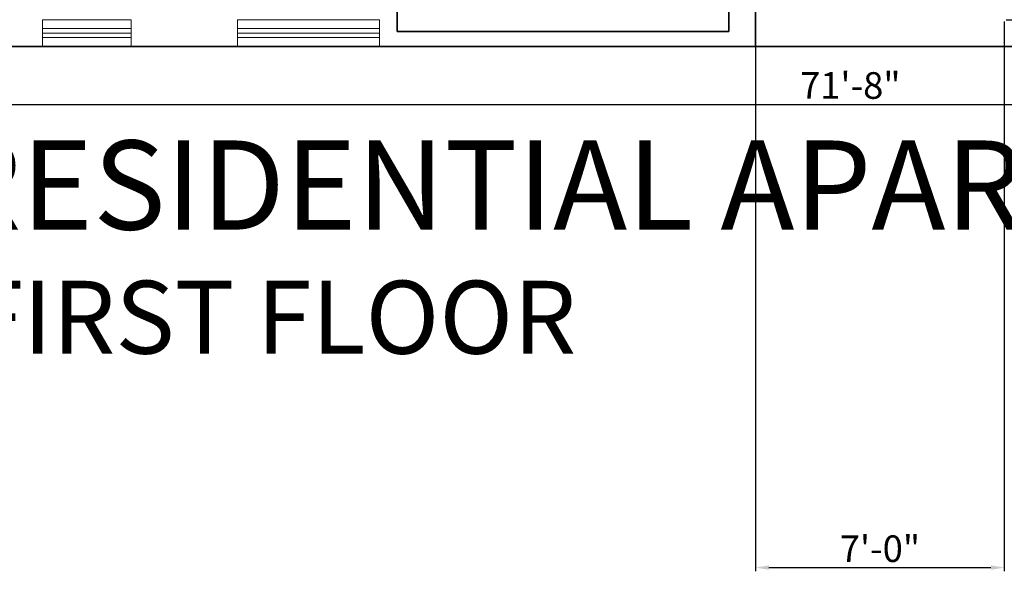
# Model space of a CAD drawing. Units: inches. Extents: x 2081 to 4786, y 1256 to 3802.
# Tile 2 of 7: x 2352 to 2685, y 1256 to 1442. Entities that reach past the tile are written whole.
import ezdxf

# ---------------------------------------------------------------- set-up
doc = ezdxf.new("R2010")
doc.units = ezdxf.units.IN
for name, color, linetype, lineweight in [('A-ANNO-DIMS', 18, 'Continuous', 18), ('A-ANNO-TITL', 18, 'Continuous', 35), ('A-GLAZ', 11, 'Continuous', 18), ('A-WALL', 7, 'Continuous', 35)]:
    doc.layers.add(name, color=color, linetype=linetype, lineweight=lineweight)
doc.styles.get("Standard").update_dxf_attribs({"font": 'arial.ttf'})
doc.dimstyles.new('ISO-25', dxfattribs={"dimtxt": 9, "dimasz": 4.5, "dimexe": 1.25, "dimexo": 0.625, "dimtad": 1, "dimdec": 0, "dimlunit": 3, "dimtxsty": 'Standard', "dimcen": 2.5, "dimadec": 0, "dimazin": 0, "dimtfac": 1, "dimtdec": 0, "dimtmove": 0, "dimatfit": 3, "dimfxl": 1, "dimarcsym": 0})

# ---------------------------------------------------------------- blocks, each defined once
blk = doc.blocks.new('*D26')
at = {"layer": 'A-ANNO-DIMS', "color": 0, "lineweight": -2, "transparency": 16777216}
for p, q in [((2202.98, 1432.55), (2202.98, 1412.32)), ((3062.98, 1432.55), (3062.98, 1412.32)), ((2207.48, 1413.57), (3058.48, 1413.57))]:
    blk.add_line(p, q, dxfattribs=at)
at = {"layer": 'A-ANNO-DIMS', "color": 0, "transparency": 16777216}
for points in [[(2207.48, 1414.32), (2207.48, 1412.82), (2202.98, 1413.57)], [(3058.48, 1414.32), (3058.48, 1412.82), (3062.98, 1413.57)]]:
    blk.add_solid(points, dxfattribs=at)
at = {"layer": 'Defpoints', "color": 0, "transparency": 16777216}
for p in [(2202.98, 1433.17), (3062.98, 1433.17), (3062.98, 1413.57)]:
    blk.add_point(p, dxfattribs=at)
at = {"layer": 'A-ANNO-DIMS', "color": 0, "transparency": 16777216, "insert": (2632.98, 1418.79), "char_height": 9, "attachment_point": 5}
blk.add_mtext('71\'-8"', dxfattribs=at)
blk = doc.blocks.new('WINDOW-48IN')
for p, q in [((0, 0), (0, 9)), ((0, 9), (4, 9)), ((4, 9), (48, 9)), ((48, 0), (48, 9)), ((48, 6), (0, 6)), ((48, 4.5), (0, 4.5)), ((48, 3), (0, 3)), ((48, 0), (0, 0))]:
    blk.add_line(p, q)
blk = doc.blocks.new('WINDOW-30IN')
for p, q in [((0, 0), (0, 30)), ((0, 30), (9, 30)), ((3, 0), (3, 30)), ((4.5, 0), (4.5, 30)), ((6, 0), (6, 30)), ((9, 30), (9, 0)), ((9, 0), (0, 0))]:
    blk.add_line(p, q)
blk = doc.blocks.new('*D80')
at = {"layer": 'A-ANNO-DIMS', "color": 0, "lineweight": -2, "transparency": 16777216}
for p, q in [((2685.61, 1484.17), (3154.73, 1484.17)), ((3153.48, 1446.67), (3153.48, 1479.67)), ((2685.61, 1442.17), (3154.73, 1442.17))]:
    blk.add_line(p, q, dxfattribs=at)
at = {"layer": 'A-ANNO-DIMS', "color": 0, "transparency": 16777216}
for points in [[(3152.73, 1479.67), (3154.23, 1479.67), (3153.48, 1484.17)], [(3152.73, 1446.67), (3154.23, 1446.67), (3153.48, 1442.17)]]:
    blk.add_solid(points, dxfattribs=at)
at = {"layer": 'Defpoints', "color": 0, "transparency": 16777216}
for p in [(2684.98, 1484.17), (3153.48, 1484.17), (2684.98, 1442.17)]:
    blk.add_point(p, dxfattribs=at)
at = {"layer": 'A-ANNO-DIMS', "color": 0, "transparency": 16777216, "insert": (3148.26, 1463.17), "char_height": 9, "attachment_point": 5, "rotation": 90}
blk.add_mtext('3\'-6"', dxfattribs=at)
blk = doc.blocks.new('*D82')
at = {"layer": 'A-ANNO-DIMS', "color": 0, "lineweight": -2, "transparency": 16777216}
for p, q in [((2600.98, 1441.55), (2600.98, 1255.85)), ((2684.98, 1441.55), (2684.98, 1255.85)), ((2605.48, 1257.1), (2680.48, 1257.1))]:
    blk.add_line(p, q, dxfattribs=at)
at = {"layer": 'A-ANNO-DIMS', "color": 0, "transparency": 16777216}
for points in [[(2605.48, 1257.85), (2605.48, 1256.35), (2600.98, 1257.1)], [(2680.48, 1257.85), (2680.48, 1256.35), (2684.98, 1257.1)]]:
    blk.add_solid(points, dxfattribs=at)
at = {"layer": 'Defpoints', "color": 0, "transparency": 16777216}
for p in [(2600.98, 1442.17), (2684.98, 1442.17), (2684.98, 1257.1)]:
    blk.add_point(p, dxfattribs=at)
at = {"layer": 'A-ANNO-DIMS', "color": 0, "transparency": 16777216, "insert": (2642.98, 1262.32), "char_height": 9, "attachment_point": 5}
blk.add_mtext('7\'-0"', dxfattribs=at)

msp = doc.modelspace()

# ---------------------------------------------------------------- linework, layer by layer
at = {"layer": 'A-WALL'}
for p, q in [((2600.98, 1433.17), (2600.98, 1780.17)), ((2479.98, 1438.17), (2479.98, 1498.17)), ((2591.98, 1438.17), (2591.98, 1498.17)), ((2591.98, 1438.17), (2479.98, 1438.17)), ((3062.98, 1433.17), (2202.98, 1433.17))]:
    msp.add_line(p, q, dxfattribs=at)

# ---------------------------------------------------------------- block references
at = {"layer": 'A-GLAZ', "rotation": 270.0000000000024}
msp.add_blockref('WINDOW-30IN', (2360.18, 1442.17), dxfattribs=at)
at = {"layer": 'A-GLAZ'}
msp.add_blockref('WINDOW-48IN', (2426.04, 1433.17), dxfattribs=at)

# ---------------------------------------------------------------- texts
at = {"layer": 'A-ANNO-TITL'}
for s, height, p in [('RESIDENTIAL APARTMENT', 30.1152, (2327.01, 1371.26)), ('FIRST FLOOR ', 24.6271, (2335.08, 1329.36))]:
    msp.add_text(s, height=height, dxfattribs=at).set_placement(p)

# ---------------------------------------------------------------- dimensions: what is measured, and where the dimension line sits
at = {"layer": 'A-ANNO-DIMS'}
dim = msp.add_linear_dim(base=(3153.48, 1484.17), p1=(2684.98, 1442.17), p2=(2684.98, 1484.17), angle=90, dimstyle='ISO-25', override={"dimdec": 1, "dimlfac": 1, "dimrnd": 0, "dimzin": 1, "dimdsep": 46, "dimlunit": 4, "dimfrac": 2}, dxfattribs=at)
dim.commit()
dim.dimension.update_dxf_attribs({"geometry": '*D80', "text_midpoint": (3148.26, 1463.17)})
for base, p1, p2, override, picture, middle in [((2684.98, 1257.1), (2600.98, 1442.17), (2684.98, 1442.17), {"dimdec": 1, "dimlfac": 1, "dimrnd": 0, "dimzin": 1, "dimdsep": 46, "dimlunit": 4, "dimfrac": 2}, '*D82', (2642.98, 1262.32)), ((3062.98, 1413.57), (2202.98, 1433.17), (3062.98, 1433.17), {"dimclrd": 0, "dimclre": 0, "dimclrt": 0}, '*D26', (2632.98, 1418.79))]:
    dim = msp.add_linear_dim(base=base, p1=p1, p2=p2, dimstyle='ISO-25', override=override, dxfattribs=at)
    dim.commit()
    dim.dimension.update_dxf_attribs({"geometry": picture, "text_midpoint": middle})

doc.saveas('drawing.dxf')
